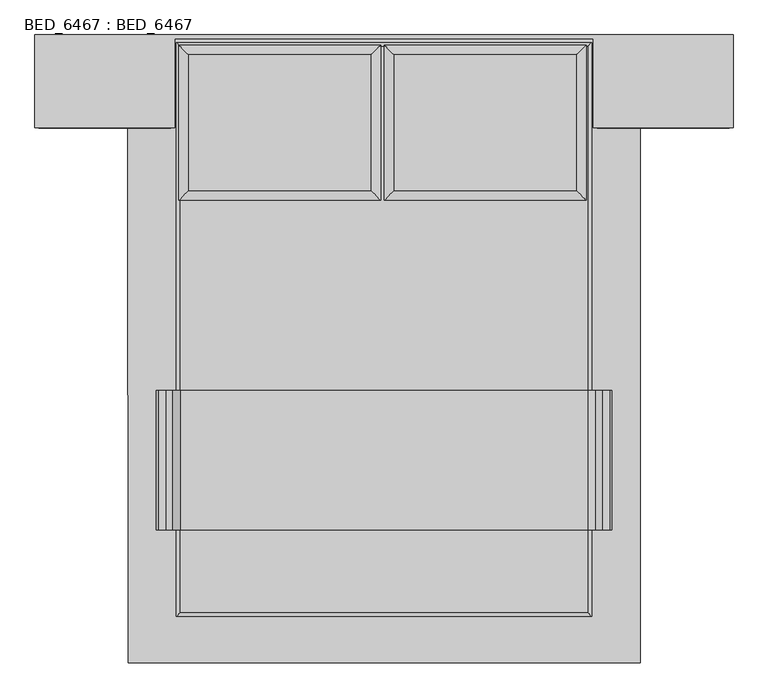
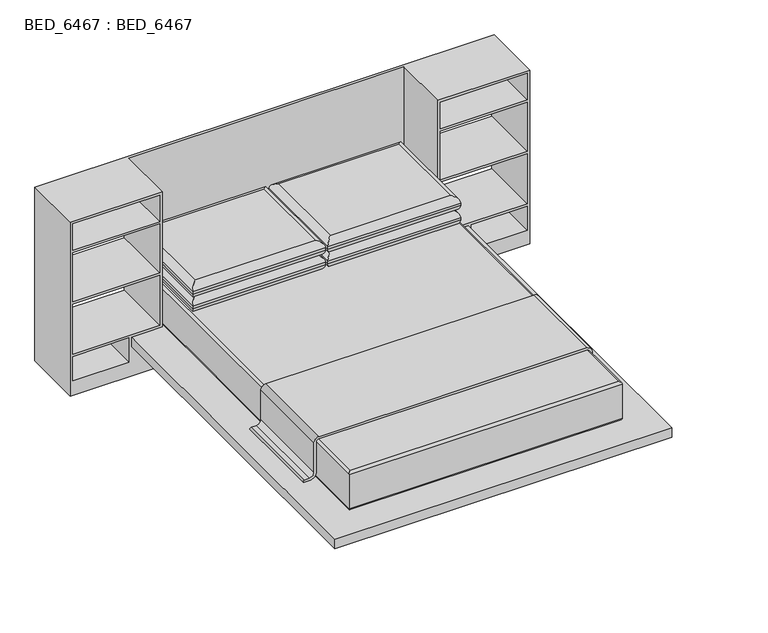
"""IFC4 building model written with IfcOpenShell, lengths in millimetres: proxy geometry, BED_6467 : BED_6467."""

from ifc_helpers import new_model, si_unit, point, frame, frame_2d, origin, place, context, project, spatial, polyline, circle_curve, ellipse_curve, trimmed, segment, composite_curve, outline, extrude, faceted_brep, source, transform, mapped, element, save
from ifc_brep_helpers import plane_surface, cylinder_surface, advanced_brep


def bed_6467_bed_6467_bd858abb(model_context):
    return source(origin(), model_context, "Body", "SolidModel", [
        advanced_brep(
        [(-695.3827629, -1070.2766054, 406.4), (638.1172371, -1070.2766054, 406.4), (638.1172371, 783.9233946, 406.4), (-695.3827629, 783.9233946, 406.4), (638.1172371, -1070.2766054, 203.2), (-695.3827629, -1070.2766054, 203.2), (-695.3827629, 783.9233946, 203.2), (638.1172371, 783.9233946, 203.2), (-708.0827629, -1082.9766054, 393.7), (-708.0827629, -1082.9766054, 215.9), (650.8172371, -1082.9766054, 215.9), (650.8172371, -1082.9766054, 393.7), (650.8172371, 796.6233946, 215.9), (650.8172371, 796.6233946, 393.7), (-708.0827629, 796.6233946, 215.9), (-708.0827629, 796.6233946, 393.7)],
        [
            (0, 1),
            (1, 2),
            (2, 3),
            (3, 0),
            (4, 5),
            (5, 6),
            (6, 7),
            (7, 4),
            (8, 9),
            (9, 10),
            (10, 11),
            (11, 8),
            (10, 12),
            (12, 13),
            (13, 11),
            (12, 14),
            (14, 15),
            (15, 13),
            (8, 15),
            (14, 9),
            (11, 1, ellipse_curve(frame((638.1172371, -1070.2766054, 393.7), z_axis=(-0.7071067811865475, -0.7071067811865475, 0.0), x_axis=(0.7071067811865476, -0.7071067811865474, 0.0)), 17.9605122, 12.7)),
            (0, 8, ellipse_curve(frame((-695.3827629, -1070.2766054, 393.7), z_axis=(0.7071067811865475, -0.7071067811865475, 0.0), x_axis=(0.7071067811865476, 0.7071067811865474, 0.0)), 17.9605122, 12.7)),
            (4, 10, ellipse_curve(frame((638.1172371, -1070.2766054, 215.9), z_axis=(-0.7071067811865475, -0.7071067811865475, 0.0), x_axis=(0.7071067811865476, -0.7071067811865474, 0.0)), 17.9605122, 12.7)),
            (9, 5, ellipse_curve(frame((-695.3827629, -1070.2766054, 215.9), z_axis=(0.7071067811865475, -0.7071067811865475, 0.0), x_axis=(0.7071067811865476, 0.7071067811865474, 0.0)), 17.9605122, 12.7)),
            (13, 2, ellipse_curve(frame((638.1172371, 783.9233946, 393.7), z_axis=(0.7071067811865475, -0.7071067811865475, 0.0), x_axis=(0.7071067811865474, 0.7071067811865476, 0.0)), 17.9605122, 12.7)),
            (7, 12, ellipse_curve(frame((638.1172371, 783.9233946, 215.9), z_axis=(0.7071067811865475, -0.7071067811865475, 0.0), x_axis=(0.7071067811865474, 0.7071067811865476, 0.0)), 17.9605122, 12.7)),
            (15, 3, ellipse_curve(frame((-695.3827629, 783.9233946, 393.7), z_axis=(0.7071067811865475, 0.7071067811865475, 0.0), x_axis=(-0.7071067811865476, 0.7071067811865474, 0.0)), 17.9605122, 12.7)),
            (6, 14, ellipse_curve(frame((-695.3827629, 783.9233946, 215.9), z_axis=(0.7071067811865475, 0.7071067811865475, 0.0), x_axis=(-0.7071067811865476, 0.7071067811865474, 0.0)), 17.9605122, 12.7)),
        ],
        [
            plane_surface(frame((-866.8327629, -1082.9766054, 406.4), z_axis=(0.0, 0.0, 1.0), x_axis=(1.0, 0.0, 0.0))),
            plane_surface(frame((-866.8327629, -1082.9766054, 203.2), z_axis=(0.0, 0.0, -1.0), x_axis=(-1.0, 0.0, 0.0))),
            plane_surface(frame((-708.0827629, -1082.9766054, 406.4), z_axis=(0.0, -1.0, 0.0), x_axis=(0.0, 0.0, -1.0))),
            plane_surface(frame((650.8172371, -1082.9766054, 406.4), z_axis=(1.0, 0.0, 0.0), x_axis=(0.0, 0.0, -1.0))),
            plane_surface(frame((650.8172371, 796.6233946, 406.4), z_axis=(0.0, 1.0, 0.0), x_axis=(0.0, 0.0, -1.0))),
            plane_surface(frame((-708.0827629, 796.6233946, 406.4), z_axis=(-1.0, 0.0, 0.0), x_axis=(0.0, 0.0, -1.0))),
            cylinder_surface(frame((-708.0827629, -1070.2766054, 393.7), z_axis=(1.0, 0.0, 0.0), x_axis=(0.0, 1.0, 0.0)), 12.7),
            cylinder_surface(frame((-708.0827629, -1070.2766054, 215.9), z_axis=(1.0, 0.0, 0.0), x_axis=(0.0, 1.0, 0.0)), 12.7),
            cylinder_surface(frame((638.1172371, -1082.9766054, 393.7), z_axis=(0.0, 1.0, 0.0), x_axis=(-1.0, 0.0, 0.0)), 12.7),
            cylinder_surface(frame((638.1172371, -1082.9766054, 215.9), z_axis=(0.0, 1.0, 0.0), x_axis=(-1.0, 0.0, 0.0)), 12.7),
            cylinder_surface(frame((650.8172371, 783.9233946, 393.7), z_axis=(-1.0, 0.0, 0.0), x_axis=(0.0, -1.0, 0.0)), 12.7),
            cylinder_surface(frame((650.8172371, 783.9233946, 215.9), z_axis=(-1.0, 0.0, 0.0), x_axis=(0.0, -1.0, 0.0)), 12.7),
            cylinder_surface(frame((-695.3827629, 796.6233946, 393.7), z_axis=(0.0, -1.0, 0.0), x_axis=(1.0, 0.0, 0.0)), 12.7),
            cylinder_surface(frame((-695.3827629, 796.6233946, 215.9), z_axis=(0.0, -1.0, 0.0), x_axis=(1.0, 0.0, 0.0)), 12.7),
        ],
        [
            (0, [[1, 2, 3, 4]]),
            (1, [[5, 6, 7, 8]]),
            (2, [[9, 10, 11, 12]]),
            (3, [[-11, 13, 14, 15]]),
            (4, [[-14, 16, 17, 18]]),
            (5, [[-9, 19, -17, 20]]),
            (6, [[21, -1, 22, -12]]),
            (7, [[23, -10, 24, -5]]),
            (8, [[-21, -15, 25, -2]]),
            (9, [[-23, -8, 26, -13]]),
            (10, [[-25, -18, 27, -3]]),
            (11, [[-26, -7, 28, -16]]),
            (12, [[-22, -4, -27, -19]]),
            (13, [[-24, -20, -28, -6]]),
        ],
    ),
        faceted_brep([(-714.4327629, 517.2233946, 914.4), (-714.4327629, 809.3233946, 914.4), (657.1672371, 809.3233946, 914.4), (657.1672371, 517.2233946, 914.4), (1114.3672371, 517.2233946, 914.4), (1114.3672371, 822.0233946, 914.4), (-1171.6327629, 822.0233946, 914.4), (-1171.6327629, 517.2233946, 914.4), (-714.4327629, 517.2233946, 0.0), (-1171.6327629, 517.2233946, 0.0), (-1171.6327629, 822.0233946, 0.0), (1114.3672371, 822.0233946, 0.0), (1114.3672371, 517.2233946, 0.0), (657.1672371, 517.2233946, 0.0), (657.1672371, 809.3233946, 0.0), (-714.4327629, 809.3233946, 0.0), (-714.4327629, 517.2233946, 203.2), (-714.4327629, 809.3233946, 203.2), (-714.4327629, 809.3233946, 152.4), (-714.4327629, 517.2233946, 152.4), (657.1672371, 809.3233946, 203.2), (657.1672371, 809.3233946, 152.4), (657.1672371, 517.2233946, 203.2), (657.1672371, 517.2233946, 152.4), (809.5672371, 517.2233946, 203.2), (809.5672371, 517.2233946, 152.4), (822.2672371, 517.2233946, 203.2), (1101.6672371, 517.2233946, 203.2), (1101.6672371, 517.2233946, 76.2), (822.2672371, 517.2233946, 76.2), (669.8672371, 517.2233946, 762.0), (669.8672371, 517.2233946, 901.7), (1101.6672371, 517.2233946, 901.7), (1101.6672371, 517.2233946, 762.0), (1101.6672371, 517.2233946, 479.0089549), (1101.6672371, 517.2233946, 215.9), (669.8672371, 517.2233946, 215.9), (669.8672371, 517.2233946, 479.0089549), (1101.6672371, 517.2233946, 749.3), (1101.6672371, 517.2233946, 491.7089549), (669.8672371, 517.2233946, 491.7089549), (669.8672371, 517.2233946, 749.3), (-1158.9327629, 822.0233946, 203.2), (-1158.9327629, 822.0233946, 76.2), (-879.5327629, 822.0233946, 76.2), (-879.5327629, 822.0233946, 203.2), (-1158.9327629, 822.0233946, 215.9), (-727.1327629, 822.0233946, 215.9), (-727.1327629, 822.0233946, 479.0089549), (-1158.9327629, 822.0233946, 479.0089549), (-727.1327629, 822.0233946, 901.7), (-1158.9327629, 822.0233946, 901.7), (-1158.9327629, 822.0233946, 762.0), (-727.1327629, 822.0233946, 762.0), (-1158.9327629, 822.0233946, 491.7089549), (-727.1327629, 822.0233946, 491.7089549), (-727.1327629, 822.0233946, 749.3), (-1158.9327629, 822.0233946, 749.3), (1101.6672371, 822.0233946, 203.2), (822.2672371, 822.0233946, 203.2), (822.2672371, 822.0233946, 76.2), (1101.6672371, 822.0233946, 76.2), (669.8672371, 822.0233946, 901.7), (669.8672371, 822.0233946, 762.0), (1101.6672371, 822.0233946, 762.0), (1101.6672371, 822.0233946, 901.7), (1101.6672371, 822.0233946, 215.9), (1101.6672371, 822.0233946, 479.0089549), (669.8672371, 822.0233946, 479.0089549), (669.8672371, 822.0233946, 215.9), (1101.6672371, 822.0233946, 491.7089549), (1101.6672371, 822.0233946, 749.3), (669.8672371, 822.0233946, 749.3), (669.8672371, 822.0233946, 491.7089549), (-866.8327629, 517.2233946, 152.4), (-866.8327629, 517.2233946, 203.2), (-1158.9327629, 517.2233946, 76.2), (-1158.9327629, 517.2233946, 203.2), (-879.5327629, 517.2233946, 203.2), (-879.5327629, 517.2233946, 76.2), (-727.1327629, 517.2233946, 215.9), (-1158.9327629, 517.2233946, 215.9), (-1158.9327629, 517.2233946, 479.0089549), (-727.1327629, 517.2233946, 479.0089549), (-1158.9327629, 517.2233946, 901.7), (-727.1327629, 517.2233946, 901.7), (-727.1327629, 517.2233946, 762.0), (-1158.9327629, 517.2233946, 762.0), (-727.1327629, 517.2233946, 491.7089549), (-1158.9327629, 517.2233946, 491.7089549), (-1158.9327629, 517.2233946, 749.3), (-727.1327629, 517.2233946, 749.3), (-866.8327629, -1235.3766054, 203.2), (809.5672371, -1235.3766054, 203.2), (809.5672371, -1235.3766054, 152.4), (-866.8327629, -1235.3766054, 152.4), (-562.0327629, 796.6233946, 152.4), (-562.0327629, -1006.7766054, 152.4), (504.7672371, -1006.7766054, 152.4), (504.7672371, 796.6233946, 152.4), (-562.0327629, 796.6233946, 0.0), (504.7672371, 796.6233946, 0.0), (504.7672371, -1006.7766054, 0.0), (-562.0327629, -1006.7766054, 0.0)], [[[0, 1, 2, 3, 4, 5, 6, 7]], [[8, 9, 10, 11, 12, 13, 14, 15]], [[1, 0, 16, 17]], [[8, 15, 18, 19]], [[2, 1, 17, 20]], [[15, 14, 21, 18]], [[3, 2, 20, 22]], [[14, 13, 23, 21]], [[4, 3, 22, 24, 25, 23, 13, 12], [26, 27, 28, 29], [30, 31, 32, 33], [34, 35, 36, 37], [38, 39, 40, 41]], [[5, 4, 12, 11]], [[6, 5, 11, 10], [42, 43, 44, 45], [46, 47, 48, 49], [50, 51, 52, 53], [54, 55, 56, 57], [58, 59, 60, 61], [62, 63, 64, 65], [66, 67, 68, 69], [70, 71, 72, 73]], [[7, 6, 10, 9]], [[0, 7, 9, 8, 19, 74, 75, 16], [76, 77, 78, 79], [80, 81, 82, 83], [84, 85, 86, 87], [88, 89, 90, 91]], [[75, 92, 93, 24, 22, 20, 17, 16]], [[25, 94, 95, 74, 19, 18, 21, 23], [96, 97, 98, 99]], [[92, 75, 74, 95]], [[93, 92, 95, 94]], [[24, 93, 94, 25]], [[100, 101, 102, 103]], [[100, 103, 97, 96]], [[103, 102, 98, 97]], [[102, 101, 99, 98]], [[101, 100, 96, 99]], [[76, 43, 42, 77]], [[43, 76, 79, 44]], [[44, 79, 78, 45]], [[77, 42, 45, 78]], [[84, 51, 50, 85]], [[51, 84, 87, 52]], [[52, 87, 86, 53]], [[85, 50, 53, 86]], [[80, 47, 46, 81]], [[47, 80, 83, 48]], [[48, 83, 82, 49]], [[81, 46, 49, 82]], [[88, 55, 54, 89]], [[55, 88, 91, 56]], [[56, 91, 90, 57]], [[89, 54, 57, 90]], [[26, 59, 58, 27]], [[59, 26, 29, 60]], [[60, 29, 28, 61]], [[27, 58, 61, 28]], [[30, 63, 62, 31]], [[63, 30, 33, 64]], [[64, 33, 32, 65]], [[31, 62, 65, 32]], [[34, 67, 66, 35]], [[67, 34, 37, 68]], [[68, 37, 36, 69]], [[35, 66, 69, 36]], [[38, 71, 70, 39]], [[71, 38, 41, 72]], [[72, 41, 40, 73]], [[39, 70, 73, 40]]]),
        advanced_brep(
        [(-668.444163, 311.8406819, 482.6), (-71.544163, 311.8406819, 482.6), (-71.544163, 756.3406819, 482.6), (-668.444163, 756.3406819, 482.6), (-71.544163, 311.8406819, 406.4), (-668.444163, 311.8406819, 406.4), (-668.444163, 756.3406819, 406.4), (-71.544163, 756.3406819, 406.4), (-39.794163, 788.0906819, 450.85), (-39.794163, 788.0906819, 438.15), (-700.194163, 788.0906819, 438.15), (-700.194163, 788.0906819, 450.85), (-700.194163, 280.0906819, 438.15), (-700.194163, 280.0906819, 450.85), (-39.794163, 280.0906819, 438.15), (-39.794163, 280.0906819, 450.85)],
        [
            (0, 1),
            (1, 2),
            (2, 3),
            (3, 0),
            (4, 5),
            (5, 6),
            (6, 7),
            (7, 4),
            (8, 9),
            (9, 10),
            (10, 11),
            (11, 8),
            (10, 12),
            (12, 13),
            (13, 11),
            (12, 14),
            (14, 15),
            (15, 13),
            (8, 15),
            (14, 9),
            (15, 1, ellipse_curve(frame((-71.544163, 311.8406819, 450.85), z_axis=(-0.7071067811865475, -0.7071067811865475, 0.0), x_axis=(0.7071067811865476, -0.7071067811865474, 0.0)), 44.9012806, 31.75)),
            (0, 13, ellipse_curve(frame((-668.444163, 311.8406819, 450.85), z_axis=(0.7071067811865475, -0.7071067811865475, 0.0), x_axis=(0.7071067811865476, 0.7071067811865474, 0.0)), 44.9012806, 31.75)),
            (4, 14, ellipse_curve(frame((-71.544163, 311.8406819, 438.15), z_axis=(-0.7071067811865475, -0.7071067811865475, 0.0), x_axis=(0.7071067811865476, -0.7071067811865474, 0.0)), 44.9012806, 31.75)),
            (12, 5, ellipse_curve(frame((-668.444163, 311.8406819, 438.15), z_axis=(0.7071067811865475, -0.7071067811865475, 0.0), x_axis=(0.7071067811865476, 0.7071067811865474, 0.0)), 44.9012806, 31.75)),
            (8, 2, ellipse_curve(frame((-71.544163, 756.3406819, 450.85), z_axis=(0.7071067811865475, -0.7071067811865475, 0.0), x_axis=(0.7071067811865474, 0.7071067811865476, 0.0)), 44.9012806, 31.75)),
            (7, 9, ellipse_curve(frame((-71.544163, 756.3406819, 438.15), z_axis=(0.7071067811865475, -0.7071067811865475, 0.0), x_axis=(0.7071067811865474, 0.7071067811865476, 0.0)), 44.9012806, 31.75)),
            (11, 3, ellipse_curve(frame((-668.444163, 756.3406819, 450.85), z_axis=(0.7071067811865475, 0.7071067811865475, 0.0), x_axis=(-0.7071067811865476, 0.7071067811865474, 0.0)), 44.9012806, 31.75)),
            (6, 10, ellipse_curve(frame((-668.444163, 756.3406819, 438.15), z_axis=(0.7071067811865475, 0.7071067811865475, 0.0), x_axis=(-0.7071067811865476, 0.7071067811865474, 0.0)), 44.9012806, 31.75)),
        ],
        [
            plane_surface(frame((-700.194163, 788.0906819, 482.6), z_axis=(0.0, 0.0, 1.0), x_axis=(-1.0, 0.0, 0.0))),
            plane_surface(frame((-700.194163, 788.0906819, 406.4), z_axis=(0.0, 0.0, -1.0), x_axis=(1.0, 0.0, 0.0))),
            plane_surface(frame((-39.794163, 788.0906819, 482.6), z_axis=(0.0, 1.0, 0.0), x_axis=(0.0, 0.0, -1.0))),
            plane_surface(frame((-700.194163, 788.0906819, 482.6), z_axis=(-1.0, 0.0, 0.0), x_axis=(0.0, 0.0, -1.0))),
            plane_surface(frame((-700.194163, 280.0906819, 482.6), z_axis=(0.0, -1.0, 0.0), x_axis=(0.0, 0.0, -1.0))),
            plane_surface(frame((-39.794163, 280.0906819, 482.6), z_axis=(1.0, 0.0, 0.0), x_axis=(0.0, 0.0, -1.0))),
            cylinder_surface(frame((-700.194163, 311.8406819, 450.85), z_axis=(1.0, 0.0, 0.0), x_axis=(0.0, 1.0, 0.0)), 31.75),
            cylinder_surface(frame((-700.194163, 311.8406819, 438.15), z_axis=(1.0, 0.0, 0.0), x_axis=(0.0, 1.0, 0.0)), 31.75),
            cylinder_surface(frame((-71.544163, 280.0906819, 450.85), z_axis=(0.0, 1.0, 0.0), x_axis=(-1.0, 0.0, 0.0)), 31.75),
            cylinder_surface(frame((-71.544163, 280.0906819, 438.15), z_axis=(0.0, 1.0, 0.0), x_axis=(-1.0, 0.0, 0.0)), 31.75),
            cylinder_surface(frame((-39.794163, 756.3406819, 450.85), z_axis=(-1.0, 0.0, 0.0), x_axis=(0.0, -1.0, 0.0)), 31.75),
            cylinder_surface(frame((-39.794163, 756.3406819, 438.15), z_axis=(-1.0, 0.0, 0.0), x_axis=(0.0, -1.0, 0.0)), 31.75),
            cylinder_surface(frame((-668.444163, 788.0906819, 450.85), z_axis=(0.0, -1.0, 0.0), x_axis=(1.0, 0.0, 0.0)), 31.75),
            cylinder_surface(frame((-668.444163, 788.0906819, 438.15), z_axis=(0.0, -1.0, 0.0), x_axis=(1.0, 0.0, 0.0)), 31.75),
        ],
        [
            (0, [[1, 2, 3, 4]]),
            (1, [[5, 6, 7, 8]]),
            (2, [[9, 10, 11, 12]]),
            (3, [[-11, 13, 14, 15]]),
            (4, [[-14, 16, 17, 18]]),
            (5, [[-9, 19, -17, 20]]),
            (6, [[21, -1, 22, -18]]),
            (7, [[23, -16, 24, -5]]),
            (8, [[-21, -19, 25, -2]]),
            (9, [[-23, -8, 26, -20]]),
            (10, [[-25, -12, 27, -3]]),
            (11, [[-26, -7, 28, -10]]),
            (12, [[-22, -4, -27, -15]]),
            (13, [[-24, -13, -28, -6]]),
        ],
    ),
        advanced_brep(
        [(4.655837, 311.8406819, 482.6), (601.555837, 311.8406819, 482.6), (601.555837, 756.3406819, 482.6), (4.655837, 756.3406819, 482.6), (601.555837, 311.8406819, 406.4), (4.655837, 311.8406819, 406.4), (4.655837, 756.3406819, 406.4), (601.555837, 756.3406819, 406.4), (633.305837, 788.0906819, 450.85), (633.305837, 788.0906819, 438.15), (-27.094163, 788.0906819, 438.15), (-27.094163, 788.0906819, 450.85), (-27.094163, 280.0906819, 438.15), (-27.094163, 280.0906819, 450.85), (633.305837, 280.0906819, 438.15), (633.305837, 280.0906819, 450.85)],
        [
            (0, 1),
            (1, 2),
            (2, 3),
            (3, 0),
            (4, 5),
            (5, 6),
            (6, 7),
            (7, 4),
            (8, 9),
            (9, 10),
            (10, 11),
            (11, 8),
            (10, 12),
            (12, 13),
            (13, 11),
            (12, 14),
            (14, 15),
            (15, 13),
            (8, 15),
            (14, 9),
            (15, 1, ellipse_curve(frame((601.555837, 311.8406819, 450.85), z_axis=(-0.7071067811865475, -0.7071067811865475, 0.0), x_axis=(0.7071067811865476, -0.7071067811865474, 0.0)), 44.9012806, 31.75)),
            (0, 13, ellipse_curve(frame((4.655837, 311.8406819, 450.85), z_axis=(0.7071067811865475, -0.7071067811865475, 0.0), x_axis=(0.7071067811865476, 0.7071067811865474, 0.0)), 44.9012806, 31.75)),
            (4, 14, ellipse_curve(frame((601.555837, 311.8406819, 438.15), z_axis=(-0.7071067811865475, -0.7071067811865475, 0.0), x_axis=(0.7071067811865476, -0.7071067811865474, 0.0)), 44.9012806, 31.75)),
            (12, 5, ellipse_curve(frame((4.655837, 311.8406819, 438.15), z_axis=(0.7071067811865475, -0.7071067811865475, 0.0), x_axis=(0.7071067811865476, 0.7071067811865474, 0.0)), 44.9012806, 31.75)),
            (8, 2, ellipse_curve(frame((601.555837, 756.3406819, 450.85), z_axis=(0.7071067811865475, -0.7071067811865475, 0.0), x_axis=(0.7071067811865474, 0.7071067811865476, 0.0)), 44.9012806, 31.75)),
            (7, 9, ellipse_curve(frame((601.555837, 756.3406819, 438.15), z_axis=(0.7071067811865475, -0.7071067811865475, 0.0), x_axis=(0.7071067811865474, 0.7071067811865476, 0.0)), 44.9012806, 31.75)),
            (11, 3, ellipse_curve(frame((4.655837, 756.3406819, 450.85), z_axis=(0.7071067811865475, 0.7071067811865475, 0.0), x_axis=(-0.7071067811865476, 0.7071067811865474, 0.0)), 44.9012806, 31.75)),
            (6, 10, ellipse_curve(frame((4.655837, 756.3406819, 438.15), z_axis=(0.7071067811865475, 0.7071067811865475, 0.0), x_axis=(-0.7071067811865476, 0.7071067811865474, 0.0)), 44.9012806, 31.75)),
        ],
        [
            plane_surface(frame((-27.094163, 788.0906819, 482.6), z_axis=(0.0, 0.0, 1.0), x_axis=(-1.0, 0.0, 0.0))),
            plane_surface(frame((-27.094163, 788.0906819, 406.4), z_axis=(0.0, 0.0, -1.0), x_axis=(1.0, 0.0, 0.0))),
            plane_surface(frame((633.305837, 788.0906819, 482.6), z_axis=(0.0, 1.0, 0.0), x_axis=(0.0, 0.0, -1.0))),
            plane_surface(frame((-27.094163, 788.0906819, 482.6), z_axis=(-1.0, 0.0, 0.0), x_axis=(0.0, 0.0, -1.0))),
            plane_surface(frame((-27.094163, 280.0906819, 482.6), z_axis=(0.0, -1.0, 0.0), x_axis=(0.0, 0.0, -1.0))),
            plane_surface(frame((633.305837, 280.0906819, 482.6), z_axis=(1.0, 0.0, 0.0), x_axis=(0.0, 0.0, -1.0))),
            cylinder_surface(frame((-27.094163, 311.8406819, 450.85), z_axis=(1.0, 0.0, 0.0), x_axis=(0.0, 1.0, 0.0)), 31.75),
            cylinder_surface(frame((-27.094163, 311.8406819, 438.15), z_axis=(1.0, 0.0, 0.0), x_axis=(0.0, 1.0, 0.0)), 31.75),
            cylinder_surface(frame((601.555837, 280.0906819, 450.85), z_axis=(0.0, 1.0, 0.0), x_axis=(-1.0, 0.0, 0.0)), 31.75),
            cylinder_surface(frame((601.555837, 280.0906819, 438.15), z_axis=(0.0, 1.0, 0.0), x_axis=(-1.0, 0.0, 0.0)), 31.75),
            cylinder_surface(frame((633.305837, 756.3406819, 450.85), z_axis=(-1.0, 0.0, 0.0), x_axis=(0.0, -1.0, 0.0)), 31.75),
            cylinder_surface(frame((633.305837, 756.3406819, 438.15), z_axis=(-1.0, 0.0, 0.0), x_axis=(0.0, -1.0, 0.0)), 31.75),
            cylinder_surface(frame((4.655837, 788.0906819, 450.85), z_axis=(0.0, -1.0, 0.0), x_axis=(1.0, 0.0, 0.0)), 31.75),
            cylinder_surface(frame((4.655837, 788.0906819, 438.15), z_axis=(0.0, -1.0, 0.0), x_axis=(1.0, 0.0, 0.0)), 31.75),
        ],
        [
            (0, [[1, 2, 3, 4]]),
            (1, [[5, 6, 7, 8]]),
            (2, [[9, 10, 11, 12]]),
            (3, [[-11, 13, 14, 15]]),
            (4, [[-14, 16, 17, 18]]),
            (5, [[-9, 19, -17, 20]]),
            (6, [[21, -1, 22, -18]]),
            (7, [[23, -16, 24, -5]]),
            (8, [[-21, -19, 25, -2]]),
            (9, [[-23, -8, 26, -20]]),
            (10, [[-25, -12, 27, -3]]),
            (11, [[-26, -7, 28, -10]]),
            (12, [[-22, -4, -27, -15]]),
            (13, [[-24, -13, -28, -6]]),
        ],
    ),
        advanced_brep(
        [(-668.444163, 311.8406819, 558.8), (-71.544163, 311.8406819, 558.8), (-71.544163, 756.3406819, 558.8), (-668.444163, 756.3406819, 558.8), (-71.544163, 311.8406819, 482.6), (-668.444163, 311.8406819, 482.6), (-668.444163, 756.3406819, 482.6), (-71.544163, 756.3406819, 482.6), (-39.794163, 788.0906819, 527.05), (-39.794163, 788.0906819, 514.35), (-700.194163, 788.0906819, 514.35), (-700.194163, 788.0906819, 527.05), (-700.194163, 280.0906819, 514.35), (-700.194163, 280.0906819, 527.05), (-39.794163, 280.0906819, 514.35), (-39.794163, 280.0906819, 527.05)],
        [
            (0, 1),
            (1, 2),
            (2, 3),
            (3, 0),
            (4, 5),
            (5, 6),
            (6, 7),
            (7, 4),
            (8, 9),
            (9, 10),
            (10, 11),
            (11, 8),
            (10, 12),
            (12, 13),
            (13, 11),
            (12, 14),
            (14, 15),
            (15, 13),
            (8, 15),
            (14, 9),
            (15, 1, ellipse_curve(frame((-71.544163, 311.8406819, 527.05), z_axis=(-0.7071067811865475, -0.7071067811865475, 0.0), x_axis=(0.7071067811865476, -0.7071067811865474, 0.0)), 44.9012806, 31.75)),
            (0, 13, ellipse_curve(frame((-668.444163, 311.8406819, 527.05), z_axis=(0.7071067811865475, -0.7071067811865475, 0.0), x_axis=(0.7071067811865476, 0.7071067811865474, 0.0)), 44.9012806, 31.75)),
            (4, 14, ellipse_curve(frame((-71.544163, 311.8406819, 514.35), z_axis=(-0.7071067811865475, -0.7071067811865475, 0.0), x_axis=(0.7071067811865476, -0.7071067811865474, 0.0)), 44.9012806, 31.75)),
            (12, 5, ellipse_curve(frame((-668.444163, 311.8406819, 514.35), z_axis=(0.7071067811865475, -0.7071067811865475, 0.0), x_axis=(0.7071067811865476, 0.7071067811865474, 0.0)), 44.9012806, 31.75)),
            (8, 2, ellipse_curve(frame((-71.544163, 756.3406819, 527.05), z_axis=(0.7071067811865475, -0.7071067811865475, 0.0), x_axis=(0.7071067811865474, 0.7071067811865476, 0.0)), 44.9012806, 31.75)),
            (7, 9, ellipse_curve(frame((-71.544163, 756.3406819, 514.35), z_axis=(0.7071067811865475, -0.7071067811865475, 0.0), x_axis=(0.7071067811865474, 0.7071067811865476, 0.0)), 44.9012806, 31.75)),
            (11, 3, ellipse_curve(frame((-668.444163, 756.3406819, 527.05), z_axis=(0.7071067811865475, 0.7071067811865475, 0.0), x_axis=(-0.7071067811865476, 0.7071067811865474, 0.0)), 44.9012806, 31.75)),
            (6, 10, ellipse_curve(frame((-668.444163, 756.3406819, 514.35), z_axis=(0.7071067811865475, 0.7071067811865475, 0.0), x_axis=(-0.7071067811865476, 0.7071067811865474, 0.0)), 44.9012806, 31.75)),
        ],
        [
            plane_surface(frame((-700.194163, 788.0906819, 558.8), z_axis=(0.0, 0.0, 1.0), x_axis=(-1.0, 0.0, 0.0))),
            plane_surface(frame((-700.194163, 788.0906819, 482.6), z_axis=(0.0, 0.0, -1.0), x_axis=(1.0, 0.0, 0.0))),
            plane_surface(frame((-39.794163, 788.0906819, 558.8), z_axis=(0.0, 1.0, 0.0), x_axis=(0.0, 0.0, -1.0))),
            plane_surface(frame((-700.194163, 788.0906819, 558.8), z_axis=(-1.0, 0.0, 0.0), x_axis=(0.0, 0.0, -1.0))),
            plane_surface(frame((-700.194163, 280.0906819, 558.8), z_axis=(0.0, -1.0, 0.0), x_axis=(0.0, 0.0, -1.0))),
            plane_surface(frame((-39.794163, 280.0906819, 558.8), z_axis=(1.0, 0.0, 0.0), x_axis=(0.0, 0.0, -1.0))),
            cylinder_surface(frame((-700.194163, 311.8406819, 527.05), z_axis=(1.0, 0.0, 0.0), x_axis=(0.0, 1.0, 0.0)), 31.75),
            cylinder_surface(frame((-700.194163, 311.8406819, 514.35), z_axis=(1.0, 0.0, 0.0), x_axis=(0.0, 1.0, 0.0)), 31.75),
            cylinder_surface(frame((-71.544163, 280.0906819, 527.05), z_axis=(0.0, 1.0, 0.0), x_axis=(-1.0, 0.0, 0.0)), 31.75),
            cylinder_surface(frame((-71.544163, 280.0906819, 514.35), z_axis=(0.0, 1.0, 0.0), x_axis=(-1.0, 0.0, 0.0)), 31.75),
            cylinder_surface(frame((-39.794163, 756.3406819, 527.05), z_axis=(-1.0, 0.0, 0.0), x_axis=(0.0, -1.0, 0.0)), 31.75),
            cylinder_surface(frame((-39.794163, 756.3406819, 514.35), z_axis=(-1.0, 0.0, 0.0), x_axis=(0.0, -1.0, 0.0)), 31.75),
            cylinder_surface(frame((-668.444163, 788.0906819, 527.05), z_axis=(0.0, -1.0, 0.0), x_axis=(1.0, 0.0, 0.0)), 31.75),
            cylinder_surface(frame((-668.444163, 788.0906819, 514.35), z_axis=(0.0, -1.0, 0.0), x_axis=(1.0, 0.0, 0.0)), 31.75),
        ],
        [
            (0, [[1, 2, 3, 4]]),
            (1, [[5, 6, 7, 8]]),
            (2, [[9, 10, 11, 12]]),
            (3, [[-11, 13, 14, 15]]),
            (4, [[-14, 16, 17, 18]]),
            (5, [[-9, 19, -17, 20]]),
            (6, [[21, -1, 22, -18]]),
            (7, [[23, -16, 24, -5]]),
            (8, [[-21, -19, 25, -2]]),
            (9, [[-23, -8, 26, -20]]),
            (10, [[-25, -12, 27, -3]]),
            (11, [[-26, -7, 28, -10]]),
            (12, [[-22, -4, -27, -15]]),
            (13, [[-24, -13, -28, -6]]),
        ],
    ),
        advanced_brep(
        [(4.655837, 311.8406819, 558.8), (601.555837, 311.8406819, 558.8), (601.555837, 756.3406819, 558.8), (4.655837, 756.3406819, 558.8), (601.555837, 311.8406819, 482.6), (4.655837, 311.8406819, 482.6), (4.655837, 756.3406819, 482.6), (601.555837, 756.3406819, 482.6), (633.305837, 788.0906819, 527.05), (633.305837, 788.0906819, 514.35), (-27.094163, 788.0906819, 514.35), (-27.094163, 788.0906819, 527.05), (-27.094163, 280.0906819, 514.35), (-27.094163, 280.0906819, 527.05), (633.305837, 280.0906819, 514.35), (633.305837, 280.0906819, 527.05)],
        [
            (0, 1),
            (1, 2),
            (2, 3),
            (3, 0),
            (4, 5),
            (5, 6),
            (6, 7),
            (7, 4),
            (8, 9),
            (9, 10),
            (10, 11),
            (11, 8),
            (10, 12),
            (12, 13),
            (13, 11),
            (12, 14),
            (14, 15),
            (15, 13),
            (8, 15),
            (14, 9),
            (15, 1, ellipse_curve(frame((601.555837, 311.8406819, 527.05), z_axis=(-0.7071067811865475, -0.7071067811865475, 0.0), x_axis=(0.7071067811865476, -0.7071067811865474, 0.0)), 44.9012806, 31.75)),
            (0, 13, ellipse_curve(frame((4.655837, 311.8406819, 527.05), z_axis=(0.7071067811865475, -0.7071067811865475, 0.0), x_axis=(0.7071067811865476, 0.7071067811865474, 0.0)), 44.9012806, 31.75)),
            (4, 14, ellipse_curve(frame((601.555837, 311.8406819, 514.35), z_axis=(-0.7071067811865475, -0.7071067811865475, 0.0), x_axis=(0.7071067811865476, -0.7071067811865474, 0.0)), 44.9012806, 31.75)),
            (12, 5, ellipse_curve(frame((4.655837, 311.8406819, 514.35), z_axis=(0.7071067811865475, -0.7071067811865475, 0.0), x_axis=(0.7071067811865476, 0.7071067811865474, 0.0)), 44.9012806, 31.75)),
            (8, 2, ellipse_curve(frame((601.555837, 756.3406819, 527.05), z_axis=(0.7071067811865475, -0.7071067811865475, 0.0), x_axis=(0.7071067811865474, 0.7071067811865476, 0.0)), 44.9012806, 31.75)),
            (7, 9, ellipse_curve(frame((601.555837, 756.3406819, 514.35), z_axis=(0.7071067811865475, -0.7071067811865475, 0.0), x_axis=(0.7071067811865474, 0.7071067811865476, 0.0)), 44.9012806, 31.75)),
            (11, 3, ellipse_curve(frame((4.655837, 756.3406819, 527.05), z_axis=(0.7071067811865475, 0.7071067811865475, 0.0), x_axis=(-0.7071067811865476, 0.7071067811865474, 0.0)), 44.9012806, 31.75)),
            (6, 10, ellipse_curve(frame((4.655837, 756.3406819, 514.35), z_axis=(0.7071067811865475, 0.7071067811865475, 0.0), x_axis=(-0.7071067811865476, 0.7071067811865474, 0.0)), 44.9012806, 31.75)),
        ],
        [
            plane_surface(frame((-27.094163, 788.0906819, 558.8), z_axis=(0.0, 0.0, 1.0), x_axis=(-1.0, 0.0, 0.0))),
            plane_surface(frame((-27.094163, 788.0906819, 482.6), z_axis=(0.0, 0.0, -1.0), x_axis=(1.0, 0.0, 0.0))),
            plane_surface(frame((633.305837, 788.0906819, 558.8), z_axis=(0.0, 1.0, 0.0), x_axis=(0.0, 0.0, -1.0))),
            plane_surface(frame((-27.094163, 788.0906819, 558.8), z_axis=(-1.0, 0.0, 0.0), x_axis=(0.0, 0.0, -1.0))),
            plane_surface(frame((-27.094163, 280.0906819, 558.8), z_axis=(0.0, -1.0, 0.0), x_axis=(0.0, 0.0, -1.0))),
            plane_surface(frame((633.305837, 280.0906819, 558.8), z_axis=(1.0, 0.0, 0.0), x_axis=(0.0, 0.0, -1.0))),
            cylinder_surface(frame((-27.094163, 311.8406819, 527.05), z_axis=(1.0, 0.0, 0.0), x_axis=(0.0, 1.0, 0.0)), 31.75),
            cylinder_surface(frame((-27.094163, 311.8406819, 514.35), z_axis=(1.0, 0.0, 0.0), x_axis=(0.0, 1.0, 0.0)), 31.75),
            cylinder_surface(frame((601.555837, 280.0906819, 527.05), z_axis=(0.0, 1.0, 0.0), x_axis=(-1.0, 0.0, 0.0)), 31.75),
            cylinder_surface(frame((601.555837, 280.0906819, 514.35), z_axis=(0.0, 1.0, 0.0), x_axis=(-1.0, 0.0, 0.0)), 31.75),
            cylinder_surface(frame((633.305837, 756.3406819, 527.05), z_axis=(-1.0, 0.0, 0.0), x_axis=(0.0, -1.0, 0.0)), 31.75),
            cylinder_surface(frame((633.305837, 756.3406819, 514.35), z_axis=(-1.0, 0.0, 0.0), x_axis=(0.0, -1.0, 0.0)), 31.75),
            cylinder_surface(frame((4.655837, 788.0906819, 527.05), z_axis=(0.0, -1.0, 0.0), x_axis=(1.0, 0.0, 0.0)), 31.75),
            cylinder_surface(frame((4.655837, 788.0906819, 514.35), z_axis=(0.0, -1.0, 0.0), x_axis=(1.0, 0.0, 0.0)), 31.75),
        ],
        [
            (0, [[1, 2, 3, 4]]),
            (1, [[5, 6, 7, 8]]),
            (2, [[9, 10, 11, 12]]),
            (3, [[-11, 13, 14, 15]]),
            (4, [[-14, 16, 17, 18]]),
            (5, [[-9, 19, -17, 20]]),
            (6, [[21, -1, 22, -18]]),
            (7, [[23, -16, 24, -5]]),
            (8, [[-21, -19, 25, -2]]),
            (9, [[-23, -8, 26, -20]]),
            (10, [[-25, -12, 27, -3]]),
            (11, [[-26, -7, 28, -10]]),
            (12, [[-22, -4, -27, -15]]),
            (13, [[-24, -13, -28, -6]]),
        ],
    ),
        extrude(outline(composite_curve([segment(trimmed(circle_curve(frame_2d((393.7, -695.3827629)), 12.7), [point((393.7, -708.0827629))], [point((406.4, -695.3827629))], True, "CARTESIAN"), True, "CONTINUOUS"), segment(polyline([(406.4, -695.3827629), (406.4, 638.1172371)]), True, "CONTINUOUS"), segment(trimmed(circle_curve(frame_2d((393.7, 638.1172371)), 12.7), [point((406.4, 638.1172371))], [point((393.7, 650.8172371))], True, "CARTESIAN"), True, "CONTINUOUS"), segment(polyline([(393.7, 650.8172371), (238.548362, 650.8172371)]), True, "CONTINUOUS"), segment(trimmed(circle_curve(frame_2d((238.548362, 686.1655991)), 35.348362), [point((238.548362, 650.8172371))], [point((203.2, 686.1655991))], False, "CARTESIAN"), True, "CONTINUOUS"), segment(polyline([(203.2, 686.1655991), (203.2, 710.6172368)]), True, "CONTINUOUS"), segment(trimmed(circle_curve(frame_2d((209.55, 710.6172368)), 6.35), [point((203.2, 710.6172368))], [point((215.9, 710.6172368))], False, "CARTESIAN"), True, "CONTINUOUS"), segment(polyline([(215.9, 710.6172368), (215.9, 686.1655991)]), True, "CONTINUOUS"), segment(trimmed(circle_curve(frame_2d((238.548362, 686.1655991)), 22.648362), [point((215.9, 686.1655991))], [point((238.548362, 663.5172371))], True, "CARTESIAN"), True, "CONTINUOUS"), segment(polyline([(238.548362, 663.5172371), (393.7, 663.5172371)]), True, "CONTINUOUS"), segment(trimmed(circle_curve(frame_2d((393.7, 638.1172371)), 25.4), [point((393.7, 663.5172371))], [point((419.1, 638.1172371))], False, "CARTESIAN"), True, "CONTINUOUS"), segment(polyline([(419.1, 638.1172371), (419.1, -695.3827629)]), True, "CONTINUOUS"), segment(trimmed(circle_curve(frame_2d((393.7, -695.3827629)), 25.4), [point((419.1, -695.3827629))], [point((393.7, -720.7827629))], False, "CARTESIAN"), True, "CONTINUOUS"), segment(polyline([(393.7, -720.7827629), (238.548362, -720.7827629)]), True, "CONTINUOUS"), segment(trimmed(circle_curve(frame_2d((238.548362, -743.4311248)), 22.648362), [point((238.548362, -720.7827629))], [point((215.9, -743.4311248))], True, "CARTESIAN"), True, "CONTINUOUS"), segment(polyline([(215.9, -743.4311248), (215.9, -767.8827625)]), True, "CONTINUOUS"), segment(trimmed(circle_curve(frame_2d((209.55, -767.8827625)), 6.35), [point((215.9, -767.8827625))], [point((203.2, -767.8827625))], False, "CARTESIAN"), True, "CONTINUOUS"), segment(polyline([(203.2, -767.8827625), (203.2, -743.4311248)]), True, "CONTINUOUS"), segment(trimmed(circle_curve(frame_2d((238.548362, -743.4311248)), 35.348362), [point((203.2, -743.4311248))], [point((238.548362, -708.0827629))], False, "CARTESIAN"), True, "CONTINUOUS"), segment(polyline([(238.548362, -708.0827629), (393.7, -708.0827629)]), True, "CONTINUOUS")], self_intersect=False)), frame((0.0, -800.4016054, 0.0), z_axis=(0.0, 1.0, 0.0), x_axis=(0.0, 0.0, 1.0)), (0.0, 0.0, 1.0), 457.2),
    ])


if __name__ == "__main__":
    model = new_model("IFC4")
    model_context = context("Model", 3, world=origin())
    ifc_project = project(units=[si_unit("LENGTHUNIT", "METRE", prefix="MILLI")], contexts=[model_context])
    site = spatial("IfcSite", under=ifc_project)
    building = spatial("IfcBuilding", under=site)
    placement = place(None, origin())
    bed_6467_bed_6467_shape = bed_6467_bed_6467_bd858abb(model_context)
    element("IfcBuildingElementProxy", 1, Name="BED_6467 : BED_6467", ObjectType="BED_6467 : BED_6467", at=placement, inside=building, context=model_context, shape_type="MappedRepresentation", body=[
        mapped(bed_6467_bed_6467_shape, transform((0.0, 0.0, 0.0), x_axis=(1.0, 0.0, 0.0), y_axis=(0.0, 1.0, 0.0), z_axis=(0.0, 0.0, 1.0))),
    ])
    save(model, "model.ifc")

# Revit data of these elements
# Type "BED_6467 : BED_6467"
#   Sheets [instance default] = Sheets
#   Pillow Set 2 [instance default] = Pillow 2
#   Pillow Set 1 [instance default] = Pillow 1
#   FRAME [instance default] = frame
#   Default Elevation = 0
# Element 1 (IfcBuildingElementProxy, "BED_6467 : BED_6467")
#   Materials on its faces: "frame", "Pillow 1", "Pillow 2", "Sheets"
# Materials
#   "Sheets": class "Fabric", colour RGB 255 255 255, transparency 0
#   "Pillow 2": class "Fabric", colour RGB 255 255 255, transparency 0
#   "Pillow 1": class "Fabric", colour RGB 0 64 128, transparency 0
#   "frame": class "Wood", colour RGB 71 38 7, transparency 0
